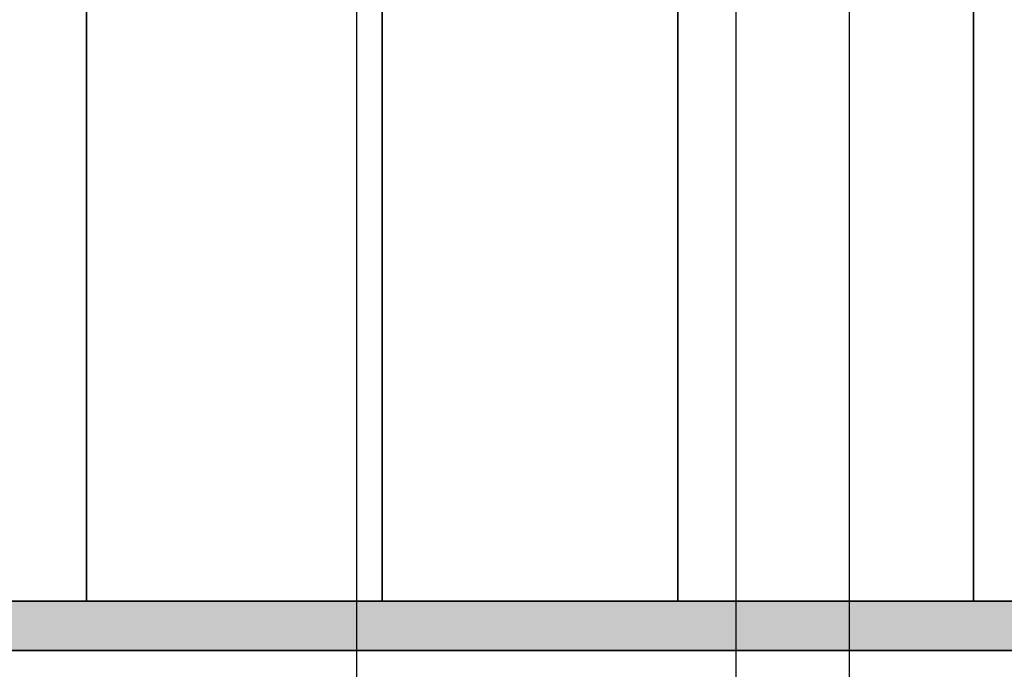
# Model space of a CAD drawing. Units: millimetres. Extents: x -22994 to 29398, y -19990 to 20176.
# Tile 30 of 135: x 119 to 139, y 30 to 43. Entities that reach past the tile are written whole.
import ezdxf
from ezdxf import colors
from ezdxf.entities.mleader import LeaderData, LeaderLine
from ezdxf.math import Vec2, Vec3

# ---------------------------------------------------------------- set-up
doc = ezdxf.new("R2010")
doc.units = ezdxf.units.MM
doc.header["$MEASUREMENT"] = 0
for name, color, linetype, lineweight in [('M-ANNO-TEXT', 7, 'Continuous', 25), ('M-DIMS', 2, 'Continuous', 18), ('M-EQPM-PATT', 7, 'Continuous', 18), ('M-PIPE', 7, 'Continuous', 35)]:
    doc.layers.add(name, color=color, linetype=linetype, lineweight=lineweight)
doc.styles.get("Standard").update_dxf_attribs({"font": 'arial.ttf'})
doc.dimstyles.get("Standard").update_dxf_attribs({"dimtxt": 0.18, "dimasz": 10000, "dimexe": 0.18, "dimexo": 0.0625, "dimgap": 0.09, "dimtad": 0, "dimtih": 1, "dimtoh": 1, "dimdec": 0, "dimzin": 0, "dimdsep": 46, "dimtxsty": 'Standard', "dimcen": 0.09, "dimadec": 0, "dimazin": 0, "dimtfac": 1, "dimtdec": 0, "dimtofl": 0, "dimtmove": 0, "dimatfit": 3, "dimfxl": 1, "dimtolj": 1, "dimtzin": 0, "dimlwd": 30, "dimarcsym": 0})

# ---------------------------------------------------------------- blocks, each defined once
blk = doc.blocks.new('*D2')
at = {"layer": 'Defpoints', "color": 0, "transparency": 16777216}
for p in [(6.677, 10.271), (290.852, 10.271), (290.852, -5.079)]:
    blk.add_point(p, dxfattribs=at)
at = {"layer": 'M-DIMS', "color": 0, "lineweight": -2, "transparency": 16777216}
for p, q in [((6.677, 10.209), (6.677, -5.259)), ((290.852, 10.209), (290.852, -5.259))]:
    blk.add_line(p, q, dxfattribs=at)
at = {"layer": 'M-DIMS', "color": 0, "lineweight": 30, "transparency": 16777216}
for p, q in [((-9993.323, -5.079), (-19993.323, -5.079)), ((10290.852, -5.079), (20290.852, -5.079))]:
    blk.add_line(p, q, dxfattribs=at)
at = {"layer": 'M-DIMS', "color": 0, "transparency": 16777216}
for points in [[(-9993.323, 1661.588), (-9993.323, -1671.745), (6.677, -5.079)], [(10290.852, 1661.588), (10290.852, -1671.745), (290.852, -5.079)]]:
    blk.add_solid(points, dxfattribs=at)
at = {"layer": 'M-DIMS', "color": 0, "transparency": 16777216, "insert": (148.765, -5.079), "char_height": 0.18, "attachment_point": 5}
blk.add_mtext('\\A1;284.2', dxfattribs=at)
blk = doc.blocks.new('*D3')
at = {"layer": 'Defpoints', "color": 0, "transparency": 16777216}
for p in [(110.265, 204.165), (110.265, 176.366), (95.833, 127.967)]:
    blk.add_point(p, dxfattribs=at)
at = {"layer": 'M-DIMS', "color": 0, "lineweight": -2, "transparency": 16777216}
for p, q in [((95.833, 128.03), (95.833, 204.345)), ((110.265, 176.429), (110.265, 204.345))]:
    blk.add_line(p, q, dxfattribs=at)
at = {"layer": 'M-DIMS', "color": 0, "lineweight": 30, "transparency": 16777216}
for p, q in [((-9904.167, 204.165), (-19904.167, 204.165)), ((10110.265, 204.165), (20110.265, 204.165))]:
    blk.add_line(p, q, dxfattribs=at)
at = {"layer": 'M-DIMS', "color": 0, "transparency": 16777216}
for points in [[(-9904.167, 1870.832), (-9904.167, -1462.501), (95.833, 204.165)], [(10110.265, 1870.832), (10110.265, -1462.501), (110.265, 204.165)]]:
    blk.add_solid(points, dxfattribs=at)
at = {"layer": 'M-DIMS', "color": 0, "transparency": 16777216, "insert": (103.049, 204.165), "char_height": 0.18, "attachment_point": 5}
blk.add_mtext('\\A1;14.432', dxfattribs=at)
blk = doc.blocks.new('*D4')
at = {"layer": 'Defpoints', "color": 0, "transparency": 16777216}
for p in [(116.265, 204.165), (110.265, 176.366), (116.265, 176.366)]:
    blk.add_point(p, dxfattribs=at)
at = {"layer": 'M-DIMS', "color": 0, "lineweight": -2, "transparency": 16777216}
for p, q in [((110.265, 176.429), (110.265, 204.345)), ((116.265, 176.429), (116.265, 204.345))]:
    blk.add_line(p, q, dxfattribs=at)
at = {"layer": 'M-DIMS', "color": 0, "lineweight": 30, "transparency": 16777216}
for p, q in [((-9889.735, 204.165), (-19889.735, 204.165)), ((10116.265, 204.165), (20116.265, 204.165))]:
    blk.add_line(p, q, dxfattribs=at)
at = {"layer": 'M-DIMS', "color": 0, "transparency": 16777216}
for points in [[(-9889.735, 1870.832), (-9889.735, -1462.501), (110.265, 204.165)], [(10116.265, 1870.832), (10116.265, -1462.501), (116.265, 204.165)]]:
    blk.add_solid(points, dxfattribs=at)
at = {"layer": 'M-DIMS', "color": 0, "transparency": 16777216, "insert": (113.265, 204.165), "char_height": 0.18, "attachment_point": 5}
blk.add_mtext('\\A1;6', dxfattribs=at)
blk = doc.blocks.new('*D5')
at = {"layer": 'Defpoints', "color": 0, "transparency": 16777216}
for p in [(181.265, 204.165), (116.265, 176.366), (181.265, 176.366)]:
    blk.add_point(p, dxfattribs=at)
at = {"layer": 'M-DIMS', "color": 0, "lineweight": -2, "transparency": 16777216}
for p, q in [((116.265, 176.429), (116.265, 204.345)), ((181.265, 176.429), (181.265, 204.345))]:
    blk.add_line(p, q, dxfattribs=at)
at = {"layer": 'M-DIMS', "color": 0, "lineweight": 30, "transparency": 16777216}
for p, q in [((-9883.735, 204.165), (-19883.735, 204.165)), ((10181.265, 204.165), (20181.265, 204.165))]:
    blk.add_line(p, q, dxfattribs=at)
at = {"layer": 'M-DIMS', "color": 0, "transparency": 16777216}
for points in [[(-9883.735, 1870.832), (-9883.735, -1462.501), (116.265, 204.165)], [(10181.265, 1870.832), (10181.265, -1462.501), (181.265, 204.165)]]:
    blk.add_solid(points, dxfattribs=at)
at = {"layer": 'M-DIMS', "color": 0, "transparency": 16777216, "insert": (148.765, 204.165), "char_height": 0.18, "attachment_point": 5}
blk.add_mtext('\\A1;65', dxfattribs=at)
blk = doc.blocks.new('*D6')
at = {"layer": 'Defpoints', "color": 0, "transparency": 16777216}
for p in [(187.265, 204.165), (181.265, 176.366), (187.265, 176.366)]:
    blk.add_point(p, dxfattribs=at)
at = {"layer": 'M-DIMS', "color": 0, "lineweight": -2, "transparency": 16777216}
for p, q in [((181.265, 176.429), (181.265, 204.345)), ((187.265, 176.429), (187.265, 204.345))]:
    blk.add_line(p, q, dxfattribs=at)
at = {"layer": 'M-DIMS', "color": 0, "lineweight": 30, "transparency": 16777216}
for p, q in [((-9818.735, 204.165), (-19818.735, 204.165)), ((10187.265, 204.165), (20187.265, 204.165))]:
    blk.add_line(p, q, dxfattribs=at)
at = {"layer": 'M-DIMS', "color": 0, "transparency": 16777216}
for points in [[(-9818.735, 1870.832), (-9818.735, -1462.501), (181.265, 204.165)], [(10187.265, 1870.832), (10187.265, -1462.501), (187.265, 204.165)]]:
    blk.add_solid(points, dxfattribs=at)
at = {"layer": 'M-DIMS', "color": 0, "transparency": 16777216, "insert": (184.265, 204.165), "char_height": 0.18, "attachment_point": 5}
blk.add_mtext('\\A1;6', dxfattribs=at)
blk = doc.blocks.new('*D7')
at = {"layer": 'Defpoints', "color": 0, "transparency": 16777216}
for p in [(201.697, 204.165), (187.265, 176.366), (201.697, 127.967)]:
    blk.add_point(p, dxfattribs=at)
at = {"layer": 'M-DIMS', "color": 0, "lineweight": -2, "transparency": 16777216}
for p, q in [((187.265, 176.429), (187.265, 204.345)), ((201.697, 128.03), (201.697, 204.345))]:
    blk.add_line(p, q, dxfattribs=at)
at = {"layer": 'M-DIMS', "color": 0, "lineweight": 30, "transparency": 16777216}
for p, q in [((-9812.735, 204.165), (-19812.735, 204.165)), ((10201.697, 204.165), (20201.697, 204.165))]:
    blk.add_line(p, q, dxfattribs=at)
at = {"layer": 'M-DIMS', "color": 0, "transparency": 16777216}
for points in [[(-9812.735, 1870.832), (-9812.735, -1462.501), (187.265, 204.165)], [(10201.697, 1870.832), (10201.697, -1462.501), (201.697, 204.165)]]:
    blk.add_solid(points, dxfattribs=at)
at = {"layer": 'M-DIMS', "color": 0, "transparency": 16777216, "insert": (194.481, 204.165), "char_height": 0.18, "attachment_point": 5}
blk.add_mtext('\\A1;14.432', dxfattribs=at)
blk = doc.blocks.new('*D8')
at = {"layer": 'Defpoints', "color": 0, "transparency": 16777216}
for p in [(227.648, 204.165), (227.648, 146.73), (201.697, 127.967)]:
    blk.add_point(p, dxfattribs=at)
at = {"layer": 'M-DIMS', "color": 0, "lineweight": -2, "transparency": 16777216}
for p, q in [((201.697, 128.03), (201.697, 204.345)), ((227.648, 146.792), (227.648, 204.345))]:
    blk.add_line(p, q, dxfattribs=at)
at = {"layer": 'M-DIMS', "color": 0, "lineweight": 30, "transparency": 16777216}
for p, q in [((-9798.303, 204.165), (-19798.303, 204.165)), ((10227.648, 204.165), (20227.648, 204.165))]:
    blk.add_line(p, q, dxfattribs=at)
at = {"layer": 'M-DIMS', "color": 0, "transparency": 16777216}
for points in [[(-9798.303, 1870.832), (-9798.303, -1462.501), (201.697, 204.165)], [(10227.648, 1870.832), (10227.648, -1462.501), (227.648, 204.165)]]:
    blk.add_solid(points, dxfattribs=at)
at = {"layer": 'M-DIMS', "color": 0, "transparency": 16777216, "insert": (214.673, 204.165), "char_height": 0.18, "attachment_point": 5}
blk.add_mtext('\\A1;25.95', dxfattribs=at)
blk = doc.blocks.new('*D9')
at = {"layer": 'Defpoints', "color": 0, "transparency": 16777216}
for p in [(187.265, 176.366), (306.202, 176.366), (290.852, 10.271)]:
    blk.add_point(p, dxfattribs=at)
at = {"layer": 'M-DIMS', "color": 0, "lineweight": 30, "transparency": 16777216}
for p, q in [((306.202, 10176.366), (306.202, 20176.366)), ((306.202, -9989.729), (306.202, -19989.729))]:
    blk.add_line(p, q, dxfattribs=at)
at = {"layer": 'M-DIMS', "color": 0, "lineweight": -2, "transparency": 16777216}
for p, q in [((187.327, 176.366), (306.382, 176.366)), ((290.915, 10.271), (306.382, 10.271))]:
    blk.add_line(p, q, dxfattribs=at)
at = {"layer": 'M-DIMS', "color": 0, "transparency": 16777216}
for points in [[(-1360.465, 10176.366), (1972.869, 10176.366), (306.202, 176.366)], [(-1360.465, -9989.729), (1972.869, -9989.729), (306.202, 10.271)]]:
    blk.add_solid(points, dxfattribs=at)
at = {"layer": 'M-DIMS', "color": 0, "transparency": 16777216, "insert": (306.202, 93.319), "char_height": 0.18, "attachment_point": 5}
blk.add_mtext('\\A1;166.1', dxfattribs=at)
blk = doc.blocks.new('*D10')
at = {"layer": 'Defpoints', "color": 0, "transparency": 16777216}
for p in [(125.65, 136.071), (133.346, 136.071), (133.346, -5.079)]:
    blk.add_point(p, dxfattribs=at)
at = {"layer": 'M-DIMS', "color": 0, "lineweight": -2, "transparency": 16777216}
for p, q in [((125.65, 136.009), (125.65, -5.259)), ((133.346, 136.009), (133.346, -5.259))]:
    blk.add_line(p, q, dxfattribs=at)
at = {"layer": 'M-DIMS', "color": 0, "lineweight": 30, "transparency": 16777216}
for p, q in [((-9874.35, -5.079), (-19874.35, -5.079)), ((10133.346, -5.079), (20133.346, -5.079))]:
    blk.add_line(p, q, dxfattribs=at)
at = {"layer": 'M-DIMS', "color": 0, "transparency": 16777216}
for points in [[(-9874.35, 1661.588), (-9874.35, -1671.745), (125.65, -5.079)], [(10133.346, 1661.588), (10133.346, -1671.745), (133.346, -5.079)]]:
    blk.add_solid(points, dxfattribs=at)
at = {"layer": 'M-DIMS', "color": 0, "transparency": 16777216, "insert": (129.498, -5.079), "char_height": 0.18, "attachment_point": 5}
blk.add_mtext('\\A1;7.696', dxfattribs=at)
blk = doc.blocks.new('*D11')
at = {"layer": 'Defpoints', "color": 0, "transparency": 16777216}
for p in [(133.346, 136.071), (135.65, 136.071), (135.65, -5.079)]:
    blk.add_point(p, dxfattribs=at)
at = {"layer": 'M-DIMS', "color": 0, "lineweight": -2, "transparency": 16777216}
for p, q in [((133.346, 136.009), (133.346, -5.259)), ((135.65, 136.009), (135.65, -5.259))]:
    blk.add_line(p, q, dxfattribs=at)
at = {"layer": 'M-DIMS', "color": 0, "lineweight": 30, "transparency": 16777216}
for p, q in [((-9866.654, -5.079), (-19866.654, -5.079)), ((10135.65, -5.079), (20135.65, -5.079))]:
    blk.add_line(p, q, dxfattribs=at)
at = {"layer": 'M-DIMS', "color": 0, "transparency": 16777216}
for points in [[(-9866.654, 1661.588), (-9866.654, -1671.745), (133.346, -5.079)], [(10135.65, 1661.588), (10135.65, -1671.745), (135.65, -5.079)]]:
    blk.add_solid(points, dxfattribs=at)
at = {"layer": 'M-DIMS', "color": 0, "transparency": 16777216, "insert": (134.498, -5.079), "char_height": 0.18, "attachment_point": 5}
blk.add_mtext('\\A1;2.304', dxfattribs=at)
blk = doc.blocks.new('*D12')
at = {"layer": 'Defpoints', "color": 0, "transparency": 16777216}
for p in [(135.65, 136.071), (145.65, 136.071), (145.65, -5.079)]:
    blk.add_point(p, dxfattribs=at)
at = {"layer": 'M-DIMS', "color": 0, "lineweight": -2, "transparency": 16777216}
for p, q in [((135.65, 136.009), (135.65, -5.259)), ((145.65, 136.009), (145.65, -5.259))]:
    blk.add_line(p, q, dxfattribs=at)
at = {"layer": 'M-DIMS', "color": 0, "lineweight": 30, "transparency": 16777216}
for p, q in [((-9864.35, -5.079), (-19864.35, -5.079)), ((10145.65, -5.079), (20145.65, -5.079))]:
    blk.add_line(p, q, dxfattribs=at)
at = {"layer": 'M-DIMS', "color": 0, "transparency": 16777216}
for points in [[(-9864.35, 1661.588), (-9864.35, -1671.745), (135.65, -5.079)], [(10145.65, 1661.588), (10145.65, -1671.745), (145.65, -5.079)]]:
    blk.add_solid(points, dxfattribs=at)
at = {"layer": 'M-DIMS', "color": 0, "transparency": 16777216, "insert": (140.65, -5.079), "char_height": 0.18, "attachment_point": 5}
blk.add_mtext('\\A1;10', dxfattribs=at)
blk = doc.blocks.new('*D13')
at = {"layer": 'Defpoints', "color": 0, "transparency": 16777216}
for p in [(145.65, 136.071), (155.65, 136.071), (155.65, -5.079)]:
    blk.add_point(p, dxfattribs=at)
at = {"layer": 'M-DIMS', "color": 0, "lineweight": -2, "transparency": 16777216}
for p, q in [((145.65, 136.009), (145.65, -5.259)), ((155.65, 136.009), (155.65, -5.259))]:
    blk.add_line(p, q, dxfattribs=at)
at = {"layer": 'M-DIMS', "color": 0, "lineweight": 30, "transparency": 16777216}
for p, q in [((-9854.35, -5.079), (-19854.35, -5.079)), ((10155.65, -5.079), (20155.65, -5.079))]:
    blk.add_line(p, q, dxfattribs=at)
at = {"layer": 'M-DIMS', "color": 0, "transparency": 16777216}
for points in [[(-9854.35, 1661.588), (-9854.35, -1671.745), (145.65, -5.079)], [(10155.65, 1661.588), (10155.65, -1671.745), (155.65, -5.079)]]:
    blk.add_solid(points, dxfattribs=at)
at = {"layer": 'M-DIMS', "color": 0, "transparency": 16777216, "insert": (150.65, -5.079), "char_height": 0.18, "attachment_point": 5}
blk.add_mtext('\\A1;10', dxfattribs=at)
blk = doc.blocks.new('*D14')
at = {"layer": 'Defpoints', "color": 0, "transparency": 16777216}
for p in [(155.65, 136.071), (165.65, 136.071), (165.65, -5.079)]:
    blk.add_point(p, dxfattribs=at)
at = {"layer": 'M-DIMS', "color": 0, "lineweight": -2, "transparency": 16777216}
for p, q in [((155.65, 136.009), (155.65, -5.259)), ((165.65, 136.009), (165.65, -5.259))]:
    blk.add_line(p, q, dxfattribs=at)
at = {"layer": 'M-DIMS', "color": 0, "lineweight": 30, "transparency": 16777216}
for p, q in [((-9844.35, -5.079), (-19844.35, -5.079)), ((10165.65, -5.079), (20165.65, -5.079))]:
    blk.add_line(p, q, dxfattribs=at)
at = {"layer": 'M-DIMS', "color": 0, "transparency": 16777216}
for points in [[(-9844.35, 1661.588), (-9844.35, -1671.745), (155.65, -5.079)], [(10165.65, 1661.588), (10165.65, -1671.745), (165.65, -5.079)]]:
    blk.add_solid(points, dxfattribs=at)
at = {"layer": 'M-DIMS', "color": 0, "transparency": 16777216, "insert": (160.65, -5.079), "char_height": 0.18, "attachment_point": 5}
blk.add_mtext('\\A1;10', dxfattribs=at)
blk = doc.blocks.new('*D15')
at = {"layer": 'Defpoints', "color": 0, "transparency": 16777216}
for p in [(173.346, 154.788), (173.346, 136.071), (306.202, 136.071)]:
    blk.add_point(p, dxfattribs=at)
at = {"layer": 'M-DIMS', "color": 0, "lineweight": 30, "transparency": 16777216}
for p, q in [((306.202, 10154.788), (306.202, 20154.788)), ((306.202, -9863.929), (306.202, -19863.929))]:
    blk.add_line(p, q, dxfattribs=at)
at = {"layer": 'M-DIMS', "color": 0, "lineweight": -2, "transparency": 16777216}
for p, q in [((173.408, 154.788), (306.382, 154.788)), ((173.408, 136.071), (306.382, 136.071))]:
    blk.add_line(p, q, dxfattribs=at)
at = {"layer": 'M-DIMS', "color": 0, "transparency": 16777216}
for points in [[(-1360.465, 10154.788), (1972.869, 10154.788), (306.202, 154.788)], [(-1360.465, -9863.929), (1972.869, -9863.929), (306.202, 136.071)]]:
    blk.add_solid(points, dxfattribs=at)
at = {"layer": 'M-DIMS', "color": 0, "transparency": 16777216, "insert": (306.202, 145.43), "char_height": 0.18, "attachment_point": 5}
blk.add_mtext('\\A1;18.717', dxfattribs=at)
blk = doc.blocks.new('*D16')
at = {"layer": 'Defpoints', "color": 0, "transparency": 16777216}
for p in [(120.17, 204.165), (110.466, 48.035), (120.17, 48.035)]:
    blk.add_point(p, dxfattribs=at)
at = {"layer": 'M-DIMS', "color": 0, "lineweight": -2, "transparency": 16777216}
for p, q in [((110.466, 48.097), (110.466, 204.345)), ((120.17, 48.097), (120.17, 204.345))]:
    blk.add_line(p, q, dxfattribs=at)
at = {"layer": 'M-DIMS', "color": 0, "lineweight": 30, "transparency": 16777216}
for p, q in [((-9889.534, 204.165), (-19889.534, 204.165)), ((10120.17, 204.165), (20120.17, 204.165))]:
    blk.add_line(p, q, dxfattribs=at)
at = {"layer": 'M-DIMS', "color": 0, "transparency": 16777216}
for points in [[(-9889.534, 1870.832), (-9889.534, -1462.501), (110.466, 204.165)], [(10120.17, 1870.832), (10120.17, -1462.501), (120.17, 204.165)]]:
    blk.add_solid(points, dxfattribs=at)
at = {"layer": 'M-DIMS', "color": 0, "transparency": 16777216, "insert": (115.318, 204.165), "char_height": 0.18, "attachment_point": 5}
blk.add_mtext('\\A1;9.704', dxfattribs=at)
blk = doc.blocks.new('*D17')
at = {"layer": 'Defpoints', "color": 0, "transparency": 16777216}
for p in [(126.17, 204.165), (120.17, 48.035), (126.17, 48.035)]:
    blk.add_point(p, dxfattribs=at)
at = {"layer": 'M-DIMS', "color": 0, "lineweight": -2, "transparency": 16777216}
for p, q in [((120.17, 48.097), (120.17, 204.345)), ((126.17, 48.097), (126.17, 204.345))]:
    blk.add_line(p, q, dxfattribs=at)
at = {"layer": 'M-DIMS', "color": 0, "lineweight": 30, "transparency": 16777216}
for p, q in [((-9879.83, 204.165), (-19879.83, 204.165)), ((10126.17, 204.165), (20126.17, 204.165))]:
    blk.add_line(p, q, dxfattribs=at)
at = {"layer": 'M-DIMS', "color": 0, "transparency": 16777216}
for points in [[(-9879.83, 1870.832), (-9879.83, -1462.501), (120.17, 204.165)], [(10126.17, 1870.832), (10126.17, -1462.501), (126.17, 204.165)]]:
    blk.add_solid(points, dxfattribs=at)
at = {"layer": 'M-DIMS', "color": 0, "transparency": 16777216, "insert": (123.17, 204.165), "char_height": 0.18, "attachment_point": 5}
blk.add_mtext('\\A1;6', dxfattribs=at)
blk = doc.blocks.new('*D18')
at = {"layer": 'Defpoints', "color": 0, "transparency": 16777216}
for p in [(132.17, 204.165), (126.17, 48.035), (132.17, 48.035)]:
    blk.add_point(p, dxfattribs=at)
at = {"layer": 'M-DIMS', "color": 0, "lineweight": -2, "transparency": 16777216}
for p, q in [((126.17, 48.097), (126.17, 204.345)), ((132.17, 48.097), (132.17, 204.345))]:
    blk.add_line(p, q, dxfattribs=at)
at = {"layer": 'M-DIMS', "color": 0, "lineweight": 30, "transparency": 16777216}
for p, q in [((-9873.83, 204.165), (-19873.83, 204.165)), ((10132.17, 204.165), (20132.17, 204.165))]:
    blk.add_line(p, q, dxfattribs=at)
at = {"layer": 'M-DIMS', "color": 0, "transparency": 16777216}
for points in [[(-9873.83, 1870.832), (-9873.83, -1462.501), (126.17, 204.165)], [(10132.17, 1870.832), (10132.17, -1462.501), (132.17, 204.165)]]:
    blk.add_solid(points, dxfattribs=at)
at = {"layer": 'M-DIMS', "color": 0, "transparency": 16777216, "insert": (129.17, 204.165), "char_height": 0.18, "attachment_point": 5}
blk.add_mtext('\\A1;6', dxfattribs=at)
blk = doc.blocks.new('*D19')
at = {"layer": 'Defpoints', "color": 0, "transparency": 16777216}
for p in [(138.17, 204.165), (132.17, 48.035), (138.17, 48.035)]:
    blk.add_point(p, dxfattribs=at)
at = {"layer": 'M-DIMS', "color": 0, "lineweight": -2, "transparency": 16777216}
for p, q in [((132.17, 48.097), (132.17, 204.345)), ((138.17, 48.097), (138.17, 204.345))]:
    blk.add_line(p, q, dxfattribs=at)
at = {"layer": 'M-DIMS', "color": 0, "lineweight": 30, "transparency": 16777216}
for p, q in [((-9867.83, 204.165), (-19867.83, 204.165)), ((10138.17, 204.165), (20138.17, 204.165))]:
    blk.add_line(p, q, dxfattribs=at)
at = {"layer": 'M-DIMS', "color": 0, "transparency": 16777216}
for points in [[(-9867.83, 1870.832), (-9867.83, -1462.501), (132.17, 204.165)], [(10138.17, 1870.832), (10138.17, -1462.501), (138.17, 204.165)]]:
    blk.add_solid(points, dxfattribs=at)
at = {"layer": 'M-DIMS', "color": 0, "transparency": 16777216, "insert": (135.17, 204.165), "char_height": 0.18, "attachment_point": 5}
blk.add_mtext('\\A1;6', dxfattribs=at)
blk = doc.blocks.new('*D20')
at = {"layer": 'Defpoints', "color": 0, "transparency": 16777216}
for p in [(144.17, 204.165), (138.17, 48.035), (144.17, 48.035)]:
    blk.add_point(p, dxfattribs=at)
at = {"layer": 'M-DIMS', "color": 0, "lineweight": -2, "transparency": 16777216}
for p, q in [((138.17, 48.097), (138.17, 204.345)), ((144.17, 48.097), (144.17, 204.345))]:
    blk.add_line(p, q, dxfattribs=at)
at = {"layer": 'M-DIMS', "color": 0, "lineweight": 30, "transparency": 16777216}
for p, q in [((-9861.83, 204.165), (-19861.83, 204.165)), ((10144.17, 204.165), (20144.17, 204.165))]:
    blk.add_line(p, q, dxfattribs=at)
at = {"layer": 'M-DIMS', "color": 0, "transparency": 16777216}
for points in [[(-9861.83, 1870.832), (-9861.83, -1462.501), (138.17, 204.165)], [(10144.17, 1870.832), (10144.17, -1462.501), (144.17, 204.165)]]:
    blk.add_solid(points, dxfattribs=at)
at = {"layer": 'M-DIMS', "color": 0, "transparency": 16777216, "insert": (141.17, 204.165), "char_height": 0.18, "attachment_point": 5}
blk.add_mtext('\\A1;6', dxfattribs=at)
blk = doc.blocks.new('*D21')
at = {"layer": 'Defpoints', "color": 0, "transparency": 16777216}
for p in [(149.116, 204.165), (144.17, 48.035), (149.116, 48.035)]:
    blk.add_point(p, dxfattribs=at)
at = {"layer": 'M-DIMS', "color": 0, "lineweight": -2, "transparency": 16777216}
for p, q in [((144.17, 48.097), (144.17, 204.345)), ((149.116, 48.097), (149.116, 204.345))]:
    blk.add_line(p, q, dxfattribs=at)
at = {"layer": 'M-DIMS', "color": 0, "lineweight": 30, "transparency": 16777216}
for p, q in [((-9855.83, 204.165), (-19855.83, 204.165)), ((10149.116, 204.165), (20149.116, 204.165))]:
    blk.add_line(p, q, dxfattribs=at)
at = {"layer": 'M-DIMS', "color": 0, "transparency": 16777216}
for points in [[(-9855.83, 1870.832), (-9855.83, -1462.501), (144.17, 204.165)], [(10149.116, 1870.832), (10149.116, -1462.501), (149.116, 204.165)]]:
    blk.add_solid(points, dxfattribs=at)
at = {"layer": 'M-DIMS', "color": 0, "transparency": 16777216, "insert": (146.643, 204.165), "char_height": 0.18, "attachment_point": 5}
blk.add_mtext('\\A1;4.945', dxfattribs=at)
blk = doc.blocks.new('*D22')
at = {"layer": 'Defpoints', "color": 0, "transparency": 16777216}
for p in [(149.116, 30.99), (155.116, 30.99), (155.116, -5.079)]:
    blk.add_point(p, dxfattribs=at)
at = {"layer": 'M-DIMS', "color": 0, "lineweight": -2, "transparency": 16777216}
for p, q in [((149.116, 30.927), (149.116, -5.259)), ((155.116, 30.927), (155.116, -5.259))]:
    blk.add_line(p, q, dxfattribs=at)
at = {"layer": 'M-DIMS', "color": 0, "lineweight": 30, "transparency": 16777216}
for p, q in [((-9850.884, -5.079), (-19850.884, -5.079)), ((10155.116, -5.079), (20155.116, -5.079))]:
    blk.add_line(p, q, dxfattribs=at)
at = {"layer": 'M-DIMS', "color": 0, "transparency": 16777216}
for points in [[(-9850.884, 1661.588), (-9850.884, -1671.745), (149.116, -5.079)], [(10155.116, 1661.588), (10155.116, -1671.745), (155.116, -5.079)]]:
    blk.add_solid(points, dxfattribs=at)
at = {"layer": 'M-DIMS', "color": 0, "transparency": 16777216, "insert": (152.116, -5.079), "char_height": 0.18, "attachment_point": 5}
blk.add_mtext('\\A1;6', dxfattribs=at)
blk = doc.blocks.new('*D23')
at = {"layer": 'Defpoints', "color": 0, "transparency": 16777216}
for p in [(155.116, 30.99), (161.116, 30.99), (161.116, -5.079)]:
    blk.add_point(p, dxfattribs=at)
at = {"layer": 'M-DIMS', "color": 0, "lineweight": -2, "transparency": 16777216}
for p, q in [((155.116, 30.927), (155.116, -5.259)), ((161.116, 30.927), (161.116, -5.259))]:
    blk.add_line(p, q, dxfattribs=at)
at = {"layer": 'M-DIMS', "color": 0, "lineweight": 30, "transparency": 16777216}
for p, q in [((-9844.884, -5.079), (-19844.884, -5.079)), ((10161.116, -5.079), (20161.116, -5.079))]:
    blk.add_line(p, q, dxfattribs=at)
at = {"layer": 'M-DIMS', "color": 0, "transparency": 16777216}
for points in [[(-9844.884, 1661.588), (-9844.884, -1671.745), (155.116, -5.079)], [(10161.116, 1661.588), (10161.116, -1671.745), (161.116, -5.079)]]:
    blk.add_solid(points, dxfattribs=at)
at = {"layer": 'M-DIMS', "color": 0, "transparency": 16777216, "insert": (158.116, -5.079), "char_height": 0.18, "attachment_point": 5}
blk.add_mtext('\\A1;6', dxfattribs=at)
blk = doc.blocks.new('*D24')
at = {"layer": 'Defpoints', "color": 0, "transparency": 16777216}
for p in [(161.116, 30.99), (166.439, 30.99), (166.439, -5.079)]:
    blk.add_point(p, dxfattribs=at)
at = {"layer": 'M-DIMS', "color": 0, "lineweight": -2, "transparency": 16777216}
for p, q in [((161.116, 30.927), (161.116, -5.259)), ((166.439, 30.927), (166.439, -5.259))]:
    blk.add_line(p, q, dxfattribs=at)
at = {"layer": 'M-DIMS', "color": 0, "lineweight": 30, "transparency": 16777216}
for p, q in [((-9838.884, -5.079), (-19838.884, -5.079)), ((10166.439, -5.079), (20166.439, -5.079))]:
    blk.add_line(p, q, dxfattribs=at)
at = {"layer": 'M-DIMS', "color": 0, "transparency": 16777216}
for points in [[(-9838.884, 1661.588), (-9838.884, -1671.745), (161.116, -5.079)], [(10166.439, 1661.588), (10166.439, -1671.745), (166.439, -5.079)]]:
    blk.add_solid(points, dxfattribs=at)
at = {"layer": 'M-DIMS', "color": 0, "transparency": 16777216, "insert": (163.777, -5.079), "char_height": 0.18, "attachment_point": 5}
blk.add_mtext('\\A1;5.323', dxfattribs=at)
blk = doc.blocks.new('*D25')
at = {"layer": 'Defpoints', "color": 0, "transparency": 16777216}
for p in [(166.439, 30.99), (172.439, 30.99), (172.439, -5.079)]:
    blk.add_point(p, dxfattribs=at)
at = {"layer": 'M-DIMS', "color": 0, "lineweight": -2, "transparency": 16777216}
for p, q in [((166.439, 30.927), (166.439, -5.259)), ((172.439, 30.927), (172.439, -5.259))]:
    blk.add_line(p, q, dxfattribs=at)
at = {"layer": 'M-DIMS', "color": 0, "lineweight": 30, "transparency": 16777216}
for p, q in [((-9833.561, -5.079), (-19833.561, -5.079)), ((10172.439, -5.079), (20172.439, -5.079))]:
    blk.add_line(p, q, dxfattribs=at)
at = {"layer": 'M-DIMS', "color": 0, "transparency": 16777216}
for points in [[(-9833.561, 1661.588), (-9833.561, -1671.745), (166.439, -5.079)], [(10172.439, 1661.588), (10172.439, -1671.745), (172.439, -5.079)]]:
    blk.add_solid(points, dxfattribs=at)
at = {"layer": 'M-DIMS', "color": 0, "transparency": 16777216, "insert": (169.439, -5.079), "char_height": 0.18, "attachment_point": 5}
blk.add_mtext('\\A1;6', dxfattribs=at)
blk = doc.blocks.new('*D26')
at = {"layer": 'Defpoints', "color": 0, "transparency": 16777216}
for p in [(172.439, 30.99), (178.439, 30.99), (178.439, -5.079)]:
    blk.add_point(p, dxfattribs=at)
at = {"layer": 'M-DIMS', "color": 0, "lineweight": -2, "transparency": 16777216}
for p, q in [((172.439, 30.927), (172.439, -5.259)), ((178.439, 30.927), (178.439, -5.259))]:
    blk.add_line(p, q, dxfattribs=at)
at = {"layer": 'M-DIMS', "color": 0, "lineweight": 30, "transparency": 16777216}
for p, q in [((-9827.561, -5.079), (-19827.561, -5.079)), ((10178.439, -5.079), (20178.439, -5.079))]:
    blk.add_line(p, q, dxfattribs=at)
at = {"layer": 'M-DIMS', "color": 0, "transparency": 16777216}
for points in [[(-9827.561, 1661.588), (-9827.561, -1671.745), (172.439, -5.079)], [(10178.439, 1661.588), (10178.439, -1671.745), (178.439, -5.079)]]:
    blk.add_solid(points, dxfattribs=at)
at = {"layer": 'M-DIMS', "color": 0, "transparency": 16777216, "insert": (175.439, -5.079), "char_height": 0.18, "attachment_point": 5}
blk.add_mtext('\\A1;6', dxfattribs=at)
blk = doc.blocks.new('*D27')
at = {"layer": 'Defpoints', "color": 0, "transparency": 16777216}
for p in [(178.439, 30.99), (188.117, 30.99), (188.117, -5.079)]:
    blk.add_point(p, dxfattribs=at)
at = {"layer": 'M-DIMS', "color": 0, "lineweight": -2, "transparency": 16777216}
for p, q in [((178.439, 30.927), (178.439, -5.259)), ((188.117, 30.927), (188.117, -5.259))]:
    blk.add_line(p, q, dxfattribs=at)
at = {"layer": 'M-DIMS', "color": 0, "lineweight": 30, "transparency": 16777216}
for p, q in [((-9821.561, -5.079), (-19821.561, -5.079)), ((10188.117, -5.079), (20188.117, -5.079))]:
    blk.add_line(p, q, dxfattribs=at)
at = {"layer": 'M-DIMS', "color": 0, "transparency": 16777216}
for points in [[(-9821.561, 1661.588), (-9821.561, -1671.745), (178.439, -5.079)], [(10188.117, 1661.588), (10188.117, -1671.745), (188.117, -5.079)]]:
    blk.add_solid(points, dxfattribs=at)
at = {"layer": 'M-DIMS', "color": 0, "transparency": 16777216, "insert": (183.278, -5.079), "char_height": 0.18, "attachment_point": 5}
blk.add_mtext('\\A1;9.679', dxfattribs=at)
blk = doc.blocks.new('*D28')
at = {"layer": 'Defpoints', "color": 0, "transparency": 16777216}
for p in [(188.117, 48.035), (306.202, 48.035), (188.117, 30.99)]:
    blk.add_point(p, dxfattribs=at)
at = {"layer": 'M-DIMS', "color": 0, "lineweight": 30, "transparency": 16777216}
for p, q in [((306.202, 10048.035), (306.202, 20048.035)), ((306.202, -9969.01), (306.202, -19969.01))]:
    blk.add_line(p, q, dxfattribs=at)
at = {"layer": 'M-DIMS', "color": 0, "lineweight": -2, "transparency": 16777216}
for p, q in [((188.18, 48.035), (306.382, 48.035)), ((188.18, 30.99), (306.382, 30.99))]:
    blk.add_line(p, q, dxfattribs=at)
at = {"layer": 'M-DIMS', "color": 0, "transparency": 16777216}
for points in [[(-1360.465, 10048.035), (1972.869, 10048.035), (306.202, 48.035)], [(-1360.465, -9969.01), (1972.869, -9969.01), (306.202, 30.99)]]:
    blk.add_solid(points, dxfattribs=at)
at = {"layer": 'M-DIMS', "color": 0, "transparency": 16777216, "insert": (306.202, 39.512), "char_height": 0.18, "attachment_point": 5}
blk.add_mtext('\\A1;17.045', dxfattribs=at)
blk = doc.blocks.new('*D29')
at = {"layer": 'Defpoints', "color": 0, "transparency": 16777216}
for p in [(36.801, 80.045), (64.03, 80.045)]:
    blk.add_point(p, dxfattribs=at)
at = {"layer": 'M-DIMS', "color": 0, "lineweight": -2, "transparency": 16777216}
for p, q in [((50.415, 79.955), (50.415, 80.135)), ((50.325, 80.045), (50.505, 80.045))]:
    blk.add_line(p, q, dxfattribs=at)
at = {"layer": 'M-DIMS', "color": 0, "lineweight": 30, "transparency": 16777216}
blk.add_line((20064.03, 80.03), (10064.03, 80.038), dxfattribs=at)
at = {"layer": 'M-DIMS', "color": 0, "transparency": 16777216}
blk.add_solid([(10064.031, 1746.704), (10064.028, -1586.629), (64.03, 80.045)], dxfattribs=at)
at = {"layer": 'M-DIMS', "color": 0, "transparency": 16777216, "insert": (20064.521, 80.03), "char_height": 0.18, "attachment_point": 5}
blk.add_mtext('\\A1;∅27.23', dxfattribs=at)
blk = doc.blocks.new('*D36')
at = {"layer": 'Defpoints', "color": 0, "transparency": 16777216}
for p in [(46.39, 31.303), (46.387, 26.593)]:
    blk.add_point(p, dxfattribs=at)
at = {"layer": 'M-DIMS', "color": 0, "lineweight": 30, "transparency": 16777216}
for p, q in [((57.15, 20031.301), (51.77, 10031.302)), ((10057.15, 20031.301), (57.15, 20031.301))]:
    blk.add_line(p, q, dxfattribs=at)
at = {"layer": 'M-DIMS', "color": 0, "lineweight": -2, "transparency": 16777216}
for p, q in [((46.389, 28.858), (46.389, 29.038)), ((46.299, 28.948), (46.479, 28.948))]:
    blk.add_line(p, q, dxfattribs=at)
at = {"layer": 'M-DIMS', "color": 0, "transparency": 16777216}
blk.add_solid([(-1614.896, 10032.199), (1718.436, 10030.405), (46.39, 31.303)], dxfattribs=at)
at = {"layer": 'M-DIMS', "color": 0, "transparency": 16777216, "insert": (10057.554, 20031.301), "char_height": 0.18, "attachment_point": 5}
blk.add_mtext('\\A1;∅4.71', dxfattribs=at)
blk = doc.blocks.new('*D37')
at = {"layer": 'Defpoints', "color": 0, "transparency": 16777216}
for p in [(54.834, 118.615), (59.494, 118.614)]:
    blk.add_point(p, dxfattribs=at)
at = {"layer": 'M-DIMS', "color": 0, "lineweight": -2, "transparency": 16777216}
for p, q in [((57.164, 118.524), (57.164, 118.704)), ((57.074, 118.614), (57.254, 118.614))]:
    blk.add_line(p, q, dxfattribs=at)
at = {"layer": 'M-DIMS', "color": 0, "lineweight": 30, "transparency": 16777216}
blk.add_line((20059.493, 116.253), (10059.494, 117.434), dxfattribs=at)
at = {"layer": 'M-DIMS', "color": 0, "transparency": 16777216}
blk.add_solid([(10059.69, 1784.1), (10059.297, -1549.233), (59.494, 118.614)], dxfattribs=at)
at = {"layer": 'M-DIMS', "color": 0, "transparency": 16777216, "insert": (20059.985, 116.253), "char_height": 0.18, "attachment_point": 5}
blk.add_mtext('\\A1;∅4.659', dxfattribs=at)

msp = doc.modelspace()

# ---------------------------------------------------------------- hatches: boundary and pattern name
at = {"layer": 'M-EQPM-PATT'}
h = msp.add_hatch(color=256, dxfattribs=at)
h.set_gradient(color1=(19, 155, 72), color2=(88, 186, 72), tint=1, name='CYLINDER')
h.paths.add_polyline_path([(109.4658, 29.9895), (189.1175, 29.9895), (189.1175, 77.6953), (128.1172, 77.6953, 0.4142136), (126.1172, 75.6953), (126.1172, 73.6953, 0.4142136), (128.1172, 71.6953), (178.5136, 71.6953, -0.4142136), (179.5136, 70.6953), (179.5136, 68.6953, -0.4142136), (178.5136, 67.6953), (128.1172, 67.6953, 0.4142136), (126.1172, 65.6953), (126.1172, 63.6953, 0.4142136), (128.1172, 61.6953), (178.5136, 61.6953, -0.4142136), (179.5136, 60.6953), (179.5136, 58.6953, -0.4142136), (178.5136, 57.6953), (109.7466, 57.6953, -0.4142136), (108.7466, 58.6953), (108.7466, 75.5922, 0.4142136), (106.7466, 77.5922), (101.8327, 77.5922), (101.8327, 76.5922), (106.7466, 76.5922, -0.4142136), (107.7466, 75.5922), (107.7466, 58.6953, 0.4142136), (109.7466, 56.6953), (178.5136, 56.6953, 0.4142136), (180.5136, 58.6953), (180.5136, 60.6953, 0.4142136), (178.5136, 62.6953), (128.1172, 62.6953, -0.4142136), (127.1172, 63.6953), (127.1172, 65.6953, -0.4142136), (128.1172, 66.6953), (178.5136, 66.6953, 0.4142136), (180.5136, 68.6953), (180.5136, 70.6953, 0.4142136), (178.5136, 72.6953), (128.1172, 72.6953, -0.4142136), (127.1172, 73.6953), (127.1172, 75.6953, -0.4142136), (128.1172, 76.6953), (188.1175, 76.6953), (188.1175, 49.0349), (110.4658, 49.0349), (110.4658, 51.9576), (101.8327, 51.9576), (101.8327, 50.9576), (109.4658, 50.9576), (109.4658, 48.5349)])
h.paths.add_polyline_path([(110.4658, 48.0349), (188.1175, 48.0349), (188.1175, 30.9895), (110.4658, 30.9895)], flags=16)
h.paths.add_polyline_path([(136.1519, 78.0082), (161.2406, 78.0082), (161.2406, 84.1903), (136.1519, 84.1903)], flags=9)

# ---------------------------------------------------------------- linework, layer by layer
at = {"layer": 'M-PIPE'}
for p, q in [((120.1702, 48.0349), (120.1702, 30.9895)), ((126.1702, 48.0349), (126.1702, 30.9895)), ((126.1702, 48.0349), (126.1702, 30.9895)), ((132.1702, 48.0349), (132.1702, 30.9895)), ((132.1702, 48.0349), (132.1702, 30.9895)), ((132.1702, 48.0349), (132.1702, 30.9895)), ((138.1702, 48.0349), (138.1702, 30.9895)), ((138.1702, 48.0349), (138.1702, 30.9895))]:
    msp.add_line(p, q, dxfattribs=at)
for points in [[(189.1175, 29.9895), (109.4658, 29.9895), (109.4658, 49.0349)], [(188.1175, 30.9895), (110.4658, 30.9895), (110.4658, 48.0349), (188.1175, 48.0349)]]:
    msp.add_lwpolyline(points, dxfattribs=at)

# ---------------------------------------------------------------- dimensions: what is measured, and where the dimension line sits
at = {"layer": 'M-DIMS'}
for base, p1, p2, override, picture, middle in [((306.202, 176.3662), (290.852, 10.2713), (187.2647, 176.3662), {"dimdec": 1, "dimlfac": 1, "dimrnd": 0, "dimzin": 0, "dimdsep": 46, "dimlunit": 2}, '*D9', (306.202, 93.3187)), ((306.202, 136.0713), (173.3459, 154.788), (173.3459, 136.0713), {"dimdec": 3, "dimlfac": 1, "dimrnd": 0, "dimzin": 0, "dimdsep": 46, "dimlunit": 2}, '*D15', (306.202, 145.4297)), ((306.202, 48.0349), (188.1175, 30.9895), (188.1175, 48.0349), {"dimdec": 3, "dimlfac": 1, "dimrnd": 0, "dimzin": 0, "dimdsep": 46, "dimlunit": 2}, '*D28', (306.202, 39.5122))]:
    dim = msp.add_linear_dim(base=base, p1=p1, p2=p2, angle=90, dimstyle='Standard', override=override, dxfattribs=at)
    dim.commit()
    dim.dimension.update_dxf_attribs({"geometry": picture, "text_midpoint": middle})
dim = msp.add_diameter_dim_2p(p1=(46.3875, 26.5934), p2=(46.39, 31.3035), dimstyle='Standard', override={"dimdec": 2, "dimlfac": 1, "dimrnd": 0, "dimzin": 0, "dimdsep": 46, "dimlunit": 2}, dxfattribs=at)
dim.commit()
dim.dimension.update_dxf_attribs({"geometry": '*D36', "text_midpoint": (10057.5542, 20031.3006), "dimtype": 163})
for base, p1, p2, override, picture, middle in [((110.2647, 204.1654), (95.8327, 127.967), (110.2647, 176.3662), {"dimdec": 3, "dimlfac": 1, "dimrnd": 0, "dimzin": 0, "dimdsep": 46, "dimlunit": 2}, '*D3', (103.0487, 204.1654)), ((116.2647, 204.1654), (110.2647, 176.3662), (116.2647, 176.3662), {"dimdec": 0, "dimlfac": 1, "dimrnd": 0, "dimzin": 0, "dimdsep": 46, "dimlunit": 2}, '*D4', (113.2647, 204.1654)), ((120.1702, 204.1654), (110.4658, 48.0349), (120.1702, 48.0349), {"dimdec": 3, "dimlfac": 1, "dimrnd": 0, "dimzin": 0, "dimdsep": 46, "dimlunit": 2}, '*D16', (115.318, 204.1654)), ((181.2647, 204.1654), (116.2647, 176.3662), (181.2647, 176.3662), {"dimdec": 0, "dimlfac": 1, "dimrnd": 0, "dimzin": 0, "dimdsep": 46, "dimlunit": 2}, '*D5', (148.7647, 204.1654)), ((126.1702, 204.1654), (120.1702, 48.0349), (126.1702, 48.0349), {"dimdec": 0, "dimlfac": 1, "dimrnd": 0, "dimzin": 0, "dimdsep": 46, "dimlunit": 2}, '*D17', (123.1702, 204.1654)), ((132.1702, 204.1654), (126.1702, 48.0349), (132.1702, 48.0349), {"dimdec": 0, "dimlfac": 1, "dimrnd": 0, "dimzin": 0, "dimdsep": 46, "dimlunit": 2}, '*D18', (129.1702, 204.1654)), ((138.1702, 204.1654), (132.1702, 48.0349), (138.1702, 48.0349), {"dimdec": 0, "dimlfac": 1, "dimrnd": 0, "dimzin": 0, "dimdsep": 46, "dimlunit": 2}, '*D19', (135.1702, 204.1654)), ((144.1702, 204.1654), (138.1702, 48.0349), (144.1702, 48.0349), {"dimdec": 0, "dimlfac": 1, "dimrnd": 0, "dimzin": 0, "dimdsep": 46, "dimlunit": 2}, '*D20', (141.1702, 204.1654)), ((149.11567, 204.16539), (144.17023, 48.03494), (149.11567, 48.03494), {"dimdec": 3, "dimlfac": 1, "dimrnd": 0, "dimzin": 0, "dimdsep": 46, "dimlunit": 2}, '*D21', (146.64295, 204.16539)), ((187.2647, 204.1654), (181.2647, 176.3662), (187.2647, 176.3662), {"dimdec": 0, "dimlfac": 1, "dimrnd": 0, "dimzin": 0, "dimdsep": 46, "dimlunit": 2}, '*D6', (184.2647, 204.1654)), ((201.6967, 204.1654), (187.2647, 176.3662), (201.6967, 127.967), {"dimdec": 3, "dimlfac": 1, "dimrnd": 0, "dimzin": 0, "dimdsep": 46, "dimlunit": 2}, '*D7', (194.4807, 204.1654)), ((227.6485, 204.1654), (201.6967, 127.967), (227.6485, 146.7296), {"dimdec": 2, "dimlfac": 1, "dimrnd": 0, "dimzin": 0, "dimdsep": 46, "dimlunit": 2}, '*D8', (214.6726, 204.1654)), ((290.852, -5.0787), (6.6773, 10.2713), (290.852, 10.2713), {"dimdec": 1, "dimlfac": 1, "dimrnd": 0, "dimzin": 0, "dimdsep": 46, "dimlunit": 2}, '*D2', (148.7647, -5.0787)), ((133.3459, -5.0787), (125.6498, 136.0713), (133.3459, 136.0713), {"dimdec": 3, "dimlfac": 1, "dimrnd": 0, "dimzin": 0, "dimdsep": 46, "dimlunit": 2}, '*D10', (129.4978, -5.0787)), ((135.6498, -5.0787), (133.3459, 136.0713), (135.6498, 136.0713), {"dimdec": 3, "dimlfac": 1, "dimrnd": 0, "dimzin": 0, "dimdsep": 46, "dimlunit": 2}, '*D11', (134.4978, -5.0787)), ((145.6498, -5.0787), (135.6498, 136.0713), (145.6498, 136.0713), {"dimdec": 0, "dimlfac": 1, "dimrnd": 0, "dimzin": 0, "dimdsep": 46, "dimlunit": 2}, '*D12', (140.6498, -5.0787)), ((155.6498, -5.0787), (145.6498, 136.0713), (155.6498, 136.0713), {"dimdec": 0, "dimlfac": 1, "dimrnd": 0, "dimzin": 0, "dimdsep": 46, "dimlunit": 2}, '*D13', (150.6498, -5.0787)), ((155.1157, -5.0787), (149.1157, 30.9895), (155.1157, 30.9895), {"dimdec": 0, "dimlfac": 1, "dimrnd": 0, "dimzin": 0, "dimdsep": 46, "dimlunit": 2}, '*D22', (152.1157, -5.0787)), ((161.1157, -5.0787), (155.1157, 30.9895), (161.1157, 30.9895), {"dimdec": 0, "dimlfac": 1, "dimrnd": 0, "dimzin": 0, "dimdsep": 46, "dimlunit": 2}, '*D23', (158.1157, -5.0787)), ((165.6498, -5.0787), (155.6498, 136.0713), (165.6498, 136.0713), {"dimdec": 0, "dimlfac": 1, "dimrnd": 0, "dimzin": 0, "dimdsep": 46, "dimlunit": 2}, '*D14', (160.6498, -5.0787)), ((166.4387, -5.0787), (161.1157, 30.9895), (166.4387, 30.9895), {"dimdec": 3, "dimlfac": 1, "dimrnd": 0, "dimzin": 0, "dimdsep": 46, "dimlunit": 2}, '*D24', (163.7772, -5.0787)), ((172.4387, -5.0787), (166.4387, 30.9895), (172.4387, 30.9895), {"dimdec": 0, "dimlfac": 1, "dimrnd": 0, "dimzin": 0, "dimdsep": 46, "dimlunit": 2}, '*D25', (169.4387, -5.0787)), ((178.4387, -5.0787), (172.4387, 30.9895), (178.4387, 30.9895), {"dimdec": 0, "dimlfac": 1, "dimrnd": 0, "dimzin": 0, "dimdsep": 46, "dimlunit": 2}, '*D26', (175.4387, -5.0787)), ((188.1175, -5.0787), (178.4387, 30.9895), (188.1175, 30.9895), {"dimdec": 3, "dimlfac": 1, "dimrnd": 0, "dimzin": 0, "dimdsep": 46, "dimlunit": 2}, '*D27', (183.2781, -5.0787))]:
    dim = msp.add_linear_dim(base=base, p1=p1, p2=p2, dimstyle='Standard', override=override, dxfattribs=at)
    dim.commit()
    dim.dimension.update_dxf_attribs({"geometry": picture, "text_midpoint": middle})
for p1, p2, override, picture, middle in [((54.8343, 118.6145), (59.4936, 118.614), {"dimdec": 3, "dimlfac": 1, "dimrnd": 0, "dimzin": 0, "dimdsep": 46, "dimlunit": 2}, '*D37', (20059.4934, 116.2531)), ((36.8006, 80.045), (64.0296, 80.045), {"dimdec": 2, "dimlfac": 1, "dimrnd": 0, "dimzin": 0, "dimdsep": 46, "dimlunit": 2}, '*D29', (20064.0296, 80.0303))]:
    dim = msp.add_diameter_dim_2p(p1=p1, p2=p2, dimstyle='Standard', override=override, dxfattribs=at)
    dim.commit()
    dim.dimension.update_dxf_attribs({"geometry": picture, "text_midpoint": middle})

# ---------------------------------------------------------------- leaders
at = {"layer": 'M-ANNO-TEXT'}
ml = msp.add_multileader_mtext('Standard', dxfattribs=at)
ml.set_content('Distributing heater', color=256)
ml.set_leader_properties()
ml.build(insert=Vec2(0, 0))
ml.multileader.update_dxf_attribs({"dogleg_length": 0.36, "arrow_head_size": 200})
ctx = ml.context
ctx.base_point, ctx.arrow_head_size, ctx.landing_gap_size, ctx.plane_origin = Vec3(86.8201, 4.9577), 200, 0.09, Vec3(80.3507, 34.8308)
notes = []
notes.append((ctx, [(1, (1, 1, 0), (82.8058, 4.9577), (1, 0), 4.0143, [(0, [(80.3507, 34.8308)], 0, [])])]))
ctx.mtext.insert, ctx.mtext.flow_direction = Vec3(86.9101, 7.5457), 5
ml = msp.add_multileader_mtext('Standard', dxfattribs=at)
ml.set_content('Circulating pump', color=256)
ml.set_leader_properties()
ml.build(insert=Vec2(0, 0))
ml.multileader.update_dxf_attribs({"dogleg_length": 0.36, "arrow_head_size": 200})
ctx = ml.context
ctx.base_point, ctx.arrow_head_size, ctx.landing_gap_size, ctx.plane_origin = Vec3(13.008, 3.5951), 200, 0.09, Vec3(56.3887, 19.3615)
ctx.text_align_type = 2
notes.append((ctx, [(1, (1, 1, 0), (63.4296, 3.5951), (-1, 0), 8.8146, [(0, [(58.1278, 30.0354)], 0, [])])]))
ctx.mtext.insert, ctx.mtext.alignment, ctx.mtext.flow_direction = Vec3(54.525, 6.1831), 3, 5
for ctx, leaders in notes:
    for number, flags, end, landing, length, lines in leaders:
        leader = LeaderData()
        leader.index, (leader.has_last_leader_line, leader.has_dogleg_vector, leader.attachment_direction) = number, flags
        leader.last_leader_point, leader.dogleg_vector, leader.dogleg_length = Vec3(end), Vec3(landing), length
        for number, points, colour, breaks in lines:
            line = LeaderLine()
            line.index, line.vertices, line.color, line.breaks = number, Vec3.list(points), colors.encode_raw_color(colour), breaks
            leader.lines.append(line)
        ctx.leaders.append(leader)

doc.saveas('drawing.dxf')
